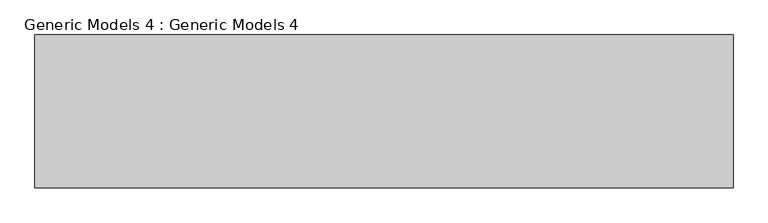
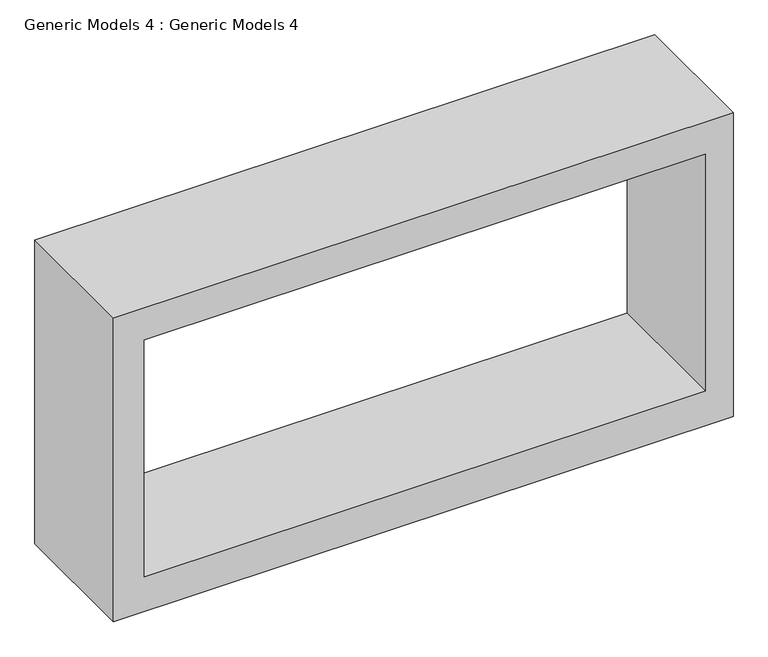
"""IFC4 building model written with IfcOpenShell, lengths in millimetres: proxy geometry, Generic Models 4 : Generic Models 4."""

from ifc_helpers import new_model, si_unit, frame, origin, place, context, project, spatial, polyline, outline, extrude, source, transform, mapped, element, save


def generic_models_4_generic_models_4_7a9117e9(model_context):
    return source(origin(), model_context, "Body", "SweptSolid", [
        extrude(outline(polyline([(6219.1316235, -3802.4859258), (6219.1316235, -8937.544821), (3555.4469154, -8937.544821), (3555.4469154, -3802.4859258), (6219.1316235, -3802.4859258)]), holes=[polyline([(5933.9332237, -8679.2859258), (5933.9332237, -4031.0859258), (3860.2469154, -4031.0859258), (3860.2469154, -8679.2859258), (5933.9332237, -8679.2859258)])]), frame((0.0, -12925.6276304, 0.0), z_axis=(0.0, 1.0, 0.0), x_axis=(0.0, 0.0, 1.0)), (0.0, 0.0, 1.0), 1124.5499072),
    ])


if __name__ == "__main__":
    model = new_model("IFC4")
    model_context = context("Model", 3, world=origin())
    ifc_project = project(units=[si_unit("LENGTHUNIT", "METRE", prefix="MILLI")], contexts=[model_context])
    site = spatial("IfcSite", under=ifc_project)
    building = spatial("IfcBuilding", under=site)
    placement = place(None, origin())
    generic_models_4_generic_models_4_shape = generic_models_4_generic_models_4_7a9117e9(model_context)
    element("IfcBuildingElementProxy", 1, Name="Generic Models 4 : Generic Models 4", ObjectType="Generic Models 4 : Generic Models 4", at=placement, inside=building, context=model_context, shape_type="MappedRepresentation", body=[
        mapped(generic_models_4_generic_models_4_shape, transform((0.0, 0.0, 0.0), x_axis=(1.0, 0.0, 0.0), y_axis=(0.0, 1.0, 0.0), z_axis=(0.0, 0.0, 1.0))),
    ])
    save(model, "model.ifc")
